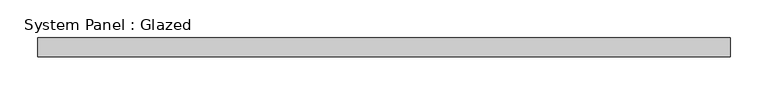
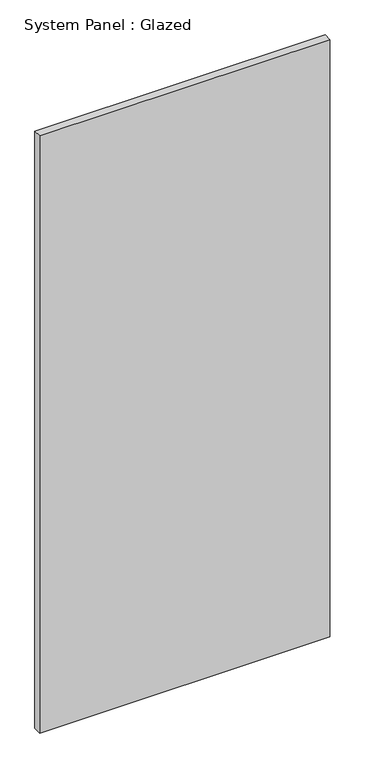
"""IFC4 building model written with IfcOpenShell, lengths in millimetres: plate geometry, System Panel : Glazed."""

from ifc_helpers import new_model, si_unit, origin, origin_with_axes, place, context, project, spatial, polyline, outline, extrude, source, transform, mapped, element, save


def system_panel_glazed_a47c5a86(model_context):
    return source(origin(), model_context, "Body", "SweptSolid", [
        extrude(outline(polyline([(460.375, 19.05), (-460.375, 19.05), (-460.375, 44.45), (460.375, 44.45), (460.375, 19.05)])), origin_with_axes(), (0.0, 0.0, 1.0), 2002.1310998),
    ])


if __name__ == "__main__":
    model = new_model("IFC4")
    model_context = context("Model", 3, world=origin())
    ifc_project = project(units=[si_unit("LENGTHUNIT", "METRE", prefix="MILLI")], contexts=[model_context])
    site = spatial("IfcSite", under=ifc_project)
    building = spatial("IfcBuilding", under=site)
    placement = place(None, origin())
    system_panel_glazed_shape = system_panel_glazed_a47c5a86(model_context)
    element("IfcPlate", 1, ObjectType="System Panel : Glazed", at=placement, inside=building, context=model_context, shape_type="MappedRepresentation", body=[
        mapped(system_panel_glazed_shape, transform((0.0, 0.0, 0.0), x_axis=(1.0, 0.0, 0.0), y_axis=(0.0, 1.0, 0.0), z_axis=(0.0, 0.0, 1.0))),
    ])
    save(model, "model.ifc")

# Revit data of these elements
# Type "System Panel : Glazed"
#   Construction Type Id = "GSP4R"
#   Analytic Construction = "1/8 in Pilkington single glazing"
#   Visual Light Transmittance = 0.9
#   Solar Heat Gain Coefficient = 0.86
#   Heat Transfer Coefficient (U) = 1.18115 BTU/(h·ft²·°F)
#   Define Thermal Properties by = 1
# Element 1 (IfcPlate, "System Panel : Glazed")
#   Materials on its faces: "Glass"
# Materials
#   "Glass": class "Glass", colour RGB 0 128 192, transparency 0.75, Description = "Soda Lime Glass", Cost = 0
